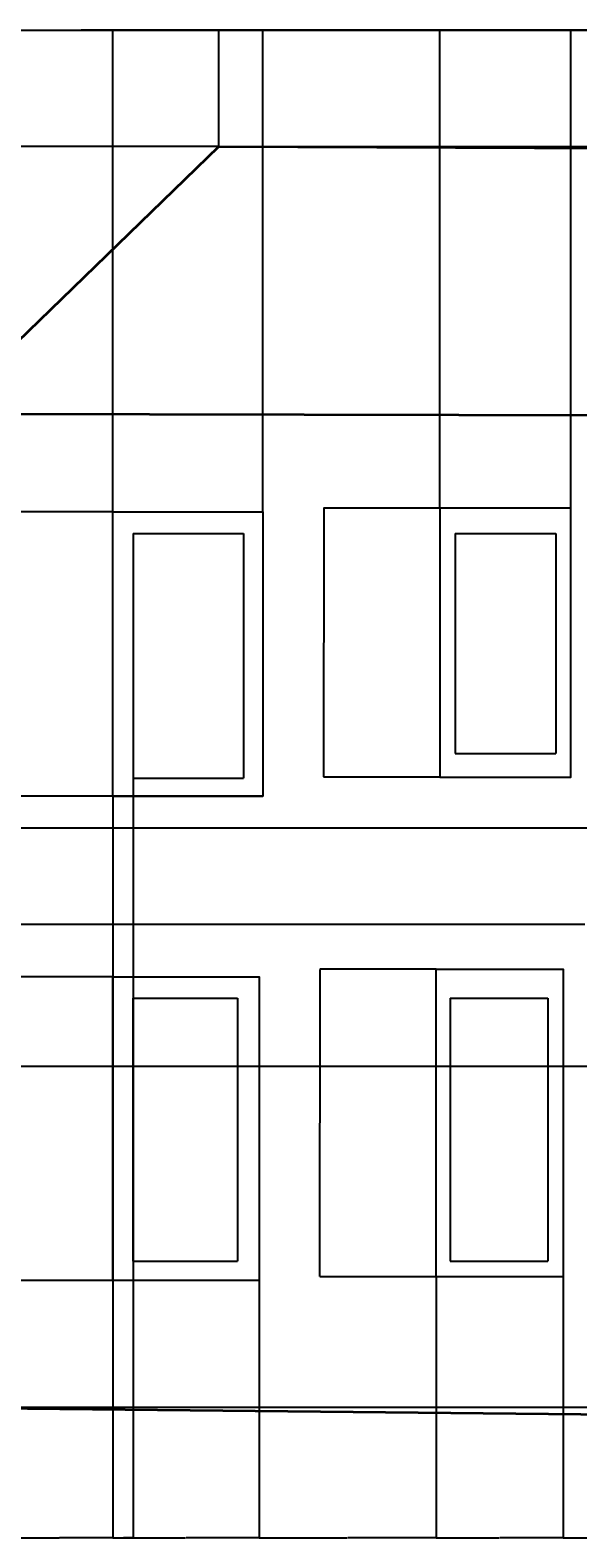
# Model space of a CAD drawing. Units: millimetres. Extents: x 1119 to 4262, y 854 to 2737.
# Tile 3 of 5: x 2434 to 3118, y 854 to 2737. Entities that reach past the tile are written whole.
import ezdxf

# ---------------------------------------------------------------- set-up
doc = ezdxf.new("R2010")
doc.units = ezdxf.units.MM
for name, color, linetype, lineweight in [('A-ANNO-DIMS', 2, 'Continuous', 18), ('A-ELEV', 8, 'Continuous', 35), ('A-GLAZ', 4, 'Continuous', 25), ('A-ROOF', 1, 'Continuous', 35)]:
    doc.layers.add(name, color=color, linetype=linetype, lineweight=lineweight)
doc.styles.get("Standard").update_dxf_attribs({"font": 'arial.ttf'})
doc.dimstyles.get("Standard").update_dxf_attribs({"dimtxt": 0.18, "dimasz": 0.18, "dimexe": 0.18, "dimexo": 0.0625, "dimgap": 0.09, "dimtad": 0, "dimtih": 1, "dimtoh": 1, "dimdec": 4, "dimzin": 0, "dimdsep": 46, "dimtxsty": 'Standard', "dimcen": 0.09, "dimadec": 0, "dimazin": 0, "dimtfac": 1, "dimtdec": 4, "dimtofl": 0, "dimtmove": 0, "dimatfit": 3, "dimfxl": 1, "dimtolj": 1, "dimtzin": 0, "dimarcsym": 0})

# ---------------------------------------------------------------- blocks, each defined once
blk = doc.blocks.new('*D5')
at = {"layer": 'A-ANNO-DIMS', "color": 0, "lineweight": -2, "transparency": 16777216}
for p, q in [((2537.2, 1175.4), (2537.2, 854.2)), ((2403.9, 1016.1), (2403.9, 854.2)), ((2404.1, 854.4), (2470.2, 854.4)), ((2537, 854.4), (2470.9, 854.4))]:
    blk.add_line(p, q, dxfattribs=at)
at = {"layer": 'A-ANNO-DIMS', "color": 0, "transparency": 16777216}
for points in [[(2404.1, 854.4), (2404.1, 854.3), (2403.9, 854.4)], [(2537, 854.4), (2537, 854.3), (2537.2, 854.4)]]:
    blk.add_solid(points, dxfattribs=at)
at = {"layer": 'Defpoints', "color": 0, "transparency": 16777216}
for p in [(2537.2, 1175.4), (2403.9, 1016.2), (2537.2, 854.4)]:
    blk.add_point(p, dxfattribs=at)
at = {"layer": 'A-ANNO-DIMS', "color": 0, "transparency": 16777216, "insert": (2470.5, 854.4), "char_height": 0.18, "attachment_point": 5}
blk.add_mtext('\\A1;133.3', dxfattribs=at)
blk = doc.blocks.new('*D6')
at = {"layer": 'A-ANNO-DIMS', "color": 0, "lineweight": -2, "transparency": 16777216}
for p, q in [((2537.2, 1175.4), (2537.2, 854.2)), ((2719.7, 1175.4), (2719.7, 854.2)), ((2537.4, 854.4), (2628, 854.4)), ((2719.5, 854.4), (2628.9, 854.4))]:
    blk.add_line(p, q, dxfattribs=at)
at = {"layer": 'A-ANNO-DIMS', "color": 0, "transparency": 16777216}
for points in [[(2537.4, 854.4), (2537.4, 854.3), (2537.2, 854.4)], [(2719.5, 854.4), (2719.5, 854.3), (2719.7, 854.4)]]:
    blk.add_solid(points, dxfattribs=at)
at = {"layer": 'Defpoints', "color": 0, "transparency": 16777216}
for p in [(2537.2, 1175.4), (2719.7, 1175.4), (2719.7, 854.4)]:
    blk.add_point(p, dxfattribs=at)
at = {"layer": 'A-ANNO-DIMS', "color": 0, "transparency": 16777216, "insert": (2628.5, 854.4), "char_height": 0.18, "attachment_point": 5}
blk.add_mtext('\\A1;182.52', dxfattribs=at)
blk = doc.blocks.new('*D7')
at = {"layer": 'A-ANNO-DIMS', "color": 0, "lineweight": -2, "transparency": 16777216}
for p, q in [((2719.7, 1175.4), (2719.7, 854.2)), ((2940.7, 1180.2), (2940.7, 854.2)), ((2719.9, 854.4), (2829.7, 854.4)), ((2940.5, 854.4), (2830.7, 854.4))]:
    blk.add_line(p, q, dxfattribs=at)
at = {"layer": 'A-ANNO-DIMS', "color": 0, "transparency": 16777216}
for points in [[(2719.9, 854.4), (2719.9, 854.3), (2719.7, 854.4)], [(2940.5, 854.4), (2940.5, 854.3), (2940.7, 854.4)]]:
    blk.add_solid(points, dxfattribs=at)
at = {"layer": 'Defpoints', "color": 0, "transparency": 16777216}
for p in [(2719.7, 1175.4), (2940.7, 1180.2), (2940.7, 854.4)]:
    blk.add_point(p, dxfattribs=at)
at = {"layer": 'A-ANNO-DIMS', "color": 0, "transparency": 16777216, "insert": (2830.2, 854.4), "char_height": 0.18, "attachment_point": 5}
blk.add_mtext('\\A1;220.95', dxfattribs=at)
blk = doc.blocks.new('*D8')
at = {"layer": 'A-ANNO-DIMS', "color": 0, "lineweight": -2, "transparency": 16777216}
for p, q in [((2940.7, 1180.2), (2940.7, 854.2)), ((3099.2, 1180.2), (3099.2, 854.2)), ((2940.8, 854.4), (3019.5, 854.4)), ((3099, 854.4), (3020.3, 854.4))]:
    blk.add_line(p, q, dxfattribs=at)
at = {"layer": 'A-ANNO-DIMS', "color": 0, "transparency": 16777216}
for points in [[(2940.8, 854.4), (2940.8, 854.3), (2940.7, 854.4)], [(3099, 854.4), (3099, 854.3), (3099.2, 854.4)]]:
    blk.add_solid(points, dxfattribs=at)
at = {"layer": 'Defpoints', "color": 0, "transparency": 16777216}
for p in [(2940.7, 1180.2), (3099.2, 1180.2), (3099.2, 854.4)]:
    blk.add_point(p, dxfattribs=at)
at = {"layer": 'A-ANNO-DIMS', "color": 0, "transparency": 16777216, "insert": (3019.9, 854.4), "char_height": 0.18, "attachment_point": 5}
blk.add_mtext('\\A1;158.5', dxfattribs=at)
blk = doc.blocks.new('*D9')
at = {"layer": 'A-ANNO-DIMS', "color": 0, "lineweight": -2, "transparency": 16777216}
for p, q in [((3099.2, 1180.2), (3099.2, 854.2)), ((3174.6, 1008), (3174.6, 854.2)), ((3099.4, 854.4), (3136.5, 854.4)), ((3174.4, 854.4), (3137.3, 854.4))]:
    blk.add_line(p, q, dxfattribs=at)
at = {"layer": 'A-ANNO-DIMS', "color": 0, "transparency": 16777216}
for points in [[(3099.4, 854.4), (3099.4, 854.3), (3099.2, 854.4)], [(3174.4, 854.4), (3174.4, 854.3), (3174.6, 854.4)]]:
    blk.add_solid(points, dxfattribs=at)
at = {"layer": 'Defpoints', "color": 0, "transparency": 16777216}
for p in [(3099.2, 1180.2), (3174.6, 1008.1), (3174.6, 854.4)]:
    blk.add_point(p, dxfattribs=at)
at = {"layer": 'A-ANNO-DIMS', "color": 0, "transparency": 16777216, "insert": (3136.9, 854.4), "char_height": 0.18, "attachment_point": 5}
blk.add_mtext('\\A1;75.38', dxfattribs=at)
blk = doc.blocks.new('*D13')
at = {"layer": 'A-ANNO-DIMS', "color": 0, "lineweight": -2, "transparency": 16777216}
for p, q in [((1264.4, 1028.3), (1264.4, 2737.1)), ((1264.5, 2737), (2690.1, 2737)), ((4116.6, 2737), (2691, 2737)), ((4116.8, 2249.8), (4116.8, 2737.1))]:
    blk.add_line(p, q, dxfattribs=at)
at = {"layer": 'A-ANNO-DIMS', "color": 0, "transparency": 16777216}
for points in [[(1264.5, 2737), (1264.5, 2736.9), (1264.4, 2737)], [(4116.6, 2737), (4116.6, 2736.9), (4116.8, 2737)]]:
    blk.add_solid(points, dxfattribs=at)
at = {"layer": 'Defpoints', "color": 0, "transparency": 16777216}
for p in [(4116.8, 2737), (4116.8, 2249.7), (1264.4, 1028.2)]:
    blk.add_point(p, dxfattribs=at)
at = {"layer": 'A-ANNO-DIMS', "color": 0, "transparency": 16777216, "insert": (2690.6, 2737), "char_height": 0.18, "attachment_point": 5}
blk.add_mtext('\\A1;2852.4', dxfattribs=at)
blk = doc.blocks.new('*D14')
at = {"layer": 'A-ANNO-DIMS', "color": 0, "lineweight": -2, "transparency": 16777216}
for p, q in [((2325.6, 2257.9), (2325.6, 2737.1)), ((2325.8, 2737), (2497.3, 2737)), ((2669.4, 2737), (2497.9, 2737)), ((2669.6, 2592), (2669.6, 2737.1))]:
    blk.add_line(p, q, dxfattribs=at)
at = {"layer": 'A-ANNO-DIMS', "color": 0, "transparency": 16777216}
for points in [[(2325.8, 2737), (2325.8, 2736.9), (2325.6, 2737)], [(2669.4, 2737), (2669.4, 2736.9), (2669.6, 2737)]]:
    blk.add_solid(points, dxfattribs=at)
at = {"layer": 'Defpoints', "color": 0, "transparency": 16777216}
for p in [(2669.6, 2737), (2669.6, 2592), (2325.6, 2257.9)]:
    blk.add_point(p, dxfattribs=at)
at = {"layer": 'A-ANNO-DIMS', "color": 0, "transparency": 16777216, "insert": (2497.6, 2737), "char_height": 0.18, "attachment_point": 5}
blk.add_mtext('\\A1;344', dxfattribs=at)
blk = doc.blocks.new('*D15')
at = {"layer": 'A-ANNO-DIMS', "color": 0, "lineweight": -2, "transparency": 16777216}
for p, q in [((2669.6, 2592), (2669.6, 2737.1)), ((2669.8, 2737), (3309.4, 2737)), ((3949.9, 2737), (3310.3, 2737)), ((3950, 2586.1), (3950, 2737.1))]:
    blk.add_line(p, q, dxfattribs=at)
at = {"layer": 'A-ANNO-DIMS', "color": 0, "transparency": 16777216}
for points in [[(2669.8, 2737), (2669.8, 2736.9), (2669.6, 2737)], [(3949.9, 2737), (3949.9, 2736.9), (3950, 2737)]]:
    blk.add_solid(points, dxfattribs=at)
at = {"layer": 'Defpoints', "color": 0, "transparency": 16777216}
for p in [(3950, 2737), (2669.6, 2592), (3950, 2586)]:
    blk.add_point(p, dxfattribs=at)
at = {"layer": 'A-ANNO-DIMS', "color": 0, "transparency": 16777216, "insert": (3309.8, 2737), "char_height": 0.18, "attachment_point": 5}
blk.add_mtext('\\A1;1280.4', dxfattribs=at)
blk = doc.blocks.new('*D25')
at = {"layer": 'A-ANNO-DIMS', "color": 0, "lineweight": -2, "transparency": 16777216}
for p, q in [((2537.2, 2135.6), (2537.2, 2737.1)), ((2537.4, 2737), (2630.4, 2737)), ((2724.3, 2737), (2631.3, 2737)), ((2724.5, 2135.6), (2724.5, 2737.1))]:
    blk.add_line(p, q, dxfattribs=at)
at = {"layer": 'A-ANNO-DIMS', "color": 0, "transparency": 16777216}
for points in [[(2537.4, 2737), (2537.4, 2736.9), (2537.2, 2737)], [(2724.3, 2737), (2724.3, 2736.9), (2724.5, 2737)]]:
    blk.add_solid(points, dxfattribs=at)
at = {"layer": 'Defpoints', "color": 0, "transparency": 16777216}
for p in [(2724.5, 2737), (2537.2, 2135.5), (2724.5, 2135.5)]:
    blk.add_point(p, dxfattribs=at)
at = {"layer": 'A-ANNO-DIMS', "color": 0, "transparency": 16777216, "insert": (2630.9, 2737), "char_height": 0.18, "attachment_point": 5}
blk.add_mtext('\\A1;187.33', dxfattribs=at)
blk = doc.blocks.new('*D26')
at = {"layer": 'A-ANNO-DIMS', "color": 0, "lineweight": -2, "transparency": 16777216}
for p, q in [((2724.5, 2135.6), (2724.5, 2737.1)), ((2724.7, 2737), (2834.5, 2737)), ((2945.3, 2737), (2835.5, 2737)), ((2945.5, 2140.4), (2945.5, 2737.1))]:
    blk.add_line(p, q, dxfattribs=at)
at = {"layer": 'A-ANNO-DIMS', "color": 0, "transparency": 16777216}
for points in [[(2724.7, 2737), (2724.7, 2736.9), (2724.5, 2737)], [(2945.3, 2737), (2945.3, 2736.9), (2945.5, 2737)]]:
    blk.add_solid(points, dxfattribs=at)
at = {"layer": 'Defpoints', "color": 0, "transparency": 16777216}
for p in [(2945.5, 2737), (2724.5, 2135.5), (2945.5, 2140.3)]:
    blk.add_point(p, dxfattribs=at)
at = {"layer": 'A-ANNO-DIMS', "color": 0, "transparency": 16777216, "insert": (2835, 2737), "char_height": 0.18, "attachment_point": 5}
blk.add_mtext('\\A1;220.95', dxfattribs=at)
blk = doc.blocks.new('*D27')
at = {"layer": 'A-ANNO-DIMS', "color": 0, "lineweight": -2, "transparency": 16777216}
for p, q in [((2945.5, 2140.4), (2945.5, 2737.1)), ((2945.6, 2737), (3026.7, 2737)), ((3108.6, 2737), (3027.5, 2737)), ((3108.8, 2140.4), (3108.8, 2737.1))]:
    blk.add_line(p, q, dxfattribs=at)
at = {"layer": 'A-ANNO-DIMS', "color": 0, "transparency": 16777216}
for points in [[(2945.6, 2737), (2945.6, 2736.9), (2945.5, 2737)], [(3108.6, 2737), (3108.6, 2736.9), (3108.8, 2737)]]:
    blk.add_solid(points, dxfattribs=at)
at = {"layer": 'Defpoints', "color": 0, "transparency": 16777216}
for p in [(3108.8, 2737), (2945.5, 2140.3), (3108.8, 2140.3)]:
    blk.add_point(p, dxfattribs=at)
at = {"layer": 'A-ANNO-DIMS', "color": 0, "transparency": 16777216, "insert": (3027.1, 2737), "char_height": 0.18, "attachment_point": 5}
blk.add_mtext('\\A1;163.3', dxfattribs=at)
blk = doc.blocks.new('*D28')
at = {"layer": 'A-ANNO-DIMS', "color": 0, "lineweight": -2, "transparency": 16777216}
for p, q in [((2562.7, 1803), (2562.7, 854.2)), ((2537.2, 1780.2), (2537.2, 854.2)), ((2537.4, 854.4), (2549.6, 854.4)), ((2562.5, 854.4), (2550.4, 854.4))]:
    blk.add_line(p, q, dxfattribs=at)
at = {"layer": 'A-ANNO-DIMS', "color": 0, "transparency": 16777216}
for points in [[(2537.4, 854.4), (2537.4, 854.3), (2537.2, 854.4)], [(2562.5, 854.4), (2562.5, 854.3), (2562.7, 854.4)]]:
    blk.add_solid(points, dxfattribs=at)
at = {"layer": 'Defpoints', "color": 0, "transparency": 16777216}
for p in [(2562.7, 1803.1), (2537.2, 1780.3), (2562.7, 854.4)]:
    blk.add_point(p, dxfattribs=at)
at = {"layer": 'A-ANNO-DIMS', "color": 0, "transparency": 16777216, "insert": (2550, 854.4), "char_height": 0.18, "attachment_point": 5}
blk.add_mtext('\\A1;25.54', dxfattribs=at)
blk = doc.blocks.new('*D29')
at = {"layer": 'A-ANNO-DIMS', "color": 0, "lineweight": -2, "transparency": 16777216}
for p, q in [((2940.6, 1564.3), (2795.5, 1564.3)), ((2795.7, 1564.1), (2795.7, 1372.4)), ((2795.7, 1180.4), (2795.7, 1372.1)), ((2940.6, 1180.2), (2795.5, 1180.2))]:
    blk.add_line(p, q, dxfattribs=at)
at = {"layer": 'A-ANNO-DIMS', "color": 0, "transparency": 16777216}
for points in [[(2795.6, 1564.1), (2795.7, 1564.1), (2795.7, 1564.3)], [(2795.6, 1180.4), (2795.7, 1180.4), (2795.7, 1180.2)]]:
    blk.add_solid(points, dxfattribs=at)
at = {"layer": 'Defpoints', "color": 0, "transparency": 16777216}
for p in [(2795.7, 1564.3), (2940.7, 1564.3), (2940.7, 1180.2)]:
    blk.add_point(p, dxfattribs=at)
at = {"layer": 'A-ANNO-DIMS', "color": 0, "transparency": 16777216, "insert": (2795.7, 1372.3), "char_height": 0.18, "attachment_point": 5}
blk.add_mtext('\\A1;384', dxfattribs=at)
blk = doc.blocks.new('*D30')
at = {"layer": 'A-ANNO-DIMS', "color": 0, "lineweight": -2, "transparency": 16777216}
for p, q in [((2945.4, 2140.3), (2800.3, 2140.3)), ((2800.5, 2140.1), (2800.5, 1972.5)), ((2800.5, 1804.5), (2800.5, 1972.1)), ((2945.4, 1804.3), (2800.3, 1804.3))]:
    blk.add_line(p, q, dxfattribs=at)
at = {"layer": 'A-ANNO-DIMS', "color": 0, "transparency": 16777216}
for points in [[(2800.4, 2140.1), (2800.5, 2140.1), (2800.5, 2140.3)], [(2800.4, 1804.5), (2800.5, 1804.5), (2800.5, 1804.3)]]:
    blk.add_solid(points, dxfattribs=at)
at = {"layer": 'Defpoints', "color": 0, "transparency": 16777216}
for p in [(2800.5, 2140.3), (2945.5, 2140.3), (2945.5, 1804.3)]:
    blk.add_point(p, dxfattribs=at)
at = {"layer": 'A-ANNO-DIMS', "color": 0, "transparency": 16777216, "insert": (2800.5, 1972.3), "char_height": 0.18, "attachment_point": 5}
blk.add_mtext('\\A1;336', dxfattribs=at)
blk = doc.blocks.new('*D31')
at = {"layer": 'A-ANNO-DIMS', "color": 0, "lineweight": -2, "transparency": 16777216}
for p, q in [((2537.1, 1175.4), (1119.2, 1175.4)), ((1119.4, 1175.3), (1119.4, 1096)), ((1119.4, 1016.4), (1119.4, 1095.6)), ((2403.8, 1016.2), (1119.2, 1016.2))]:
    blk.add_line(p, q, dxfattribs=at)
at = {"layer": 'A-ANNO-DIMS', "color": 0, "transparency": 16777216}
for points in [[(1119.3, 1175.3), (1119.4, 1175.3), (1119.4, 1175.4)], [(1119.3, 1016.4), (1119.4, 1016.4), (1119.4, 1016.2)]]:
    blk.add_solid(points, dxfattribs=at)
at = {"layer": 'Defpoints', "color": 0, "transparency": 16777216}
for p in [(1119.4, 1175.4), (2537.2, 1175.4), (2403.9, 1016.2)]:
    blk.add_point(p, dxfattribs=at)
at = {"layer": 'A-ANNO-DIMS', "color": 0, "transparency": 16777216, "insert": (1119.4, 1095.8), "char_height": 0.18, "attachment_point": 5}
blk.add_mtext('\\A1;159.26', dxfattribs=at)
blk = doc.blocks.new('*D32')
at = {"layer": 'A-ANNO-DIMS', "color": 0, "lineweight": -2, "transparency": 16777216}
for p, q in [((2537.1, 1554.7), (1119.2, 1554.7)), ((1119.4, 1554.5), (1119.4, 1365.2)), ((1119.4, 1175.6), (1119.4, 1364.9)), ((2537.1, 1175.4), (1119.2, 1175.4))]:
    blk.add_line(p, q, dxfattribs=at)
at = {"layer": 'A-ANNO-DIMS', "color": 0, "transparency": 16777216}
for points in [[(1119.3, 1554.5), (1119.4, 1554.5), (1119.4, 1554.7)], [(1119.3, 1175.6), (1119.4, 1175.6), (1119.4, 1175.4)]]:
    blk.add_solid(points, dxfattribs=at)
at = {"layer": 'Defpoints', "color": 0, "transparency": 16777216}
for p in [(1119.4, 1554.7), (2537.2, 1554.7), (2537.2, 1175.4)]:
    blk.add_point(p, dxfattribs=at)
at = {"layer": 'A-ANNO-DIMS', "color": 0, "transparency": 16777216, "insert": (1119.4, 1365.1), "char_height": 0.18, "attachment_point": 5}
blk.add_mtext('\\A1;379.2', dxfattribs=at)
blk = doc.blocks.new('*D33')
at = {"layer": 'A-ANNO-DIMS', "color": 0, "lineweight": -2, "transparency": 16777216}
for p, q in [((2537.1, 1780.3), (1119.2, 1780.3)), ((1119.4, 1780.1), (1119.4, 1667.7)), ((1119.4, 1554.9), (1119.4, 1667.3)), ((2537.1, 1554.7), (1119.2, 1554.7))]:
    blk.add_line(p, q, dxfattribs=at)
at = {"layer": 'A-ANNO-DIMS', "color": 0, "transparency": 16777216}
for points in [[(1119.3, 1780.1), (1119.4, 1780.1), (1119.4, 1780.3)], [(1119.3, 1554.9), (1119.4, 1554.9), (1119.4, 1554.7)]]:
    blk.add_solid(points, dxfattribs=at)
at = {"layer": 'Defpoints', "color": 0, "transparency": 16777216}
for p in [(1119.4, 1780.3), (2537.2, 1780.3), (2537.2, 1554.7)]:
    blk.add_point(p, dxfattribs=at)
at = {"layer": 'A-ANNO-DIMS', "color": 0, "transparency": 16777216, "insert": (1119.4, 1667.5), "char_height": 0.18, "attachment_point": 5}
blk.add_mtext('\\A1;225.6', dxfattribs=at)
blk = doc.blocks.new('*D34')
at = {"layer": 'A-ANNO-DIMS', "color": 0, "lineweight": -2, "transparency": 16777216}
for p, q in [((2537.1, 2135.5), (1119.2, 2135.5)), ((1119.4, 2135.3), (1119.4, 1958.1)), ((1119.4, 1780.5), (1119.4, 1957.7)), ((2537.1, 1780.3), (1119.2, 1780.3))]:
    blk.add_line(p, q, dxfattribs=at)
at = {"layer": 'A-ANNO-DIMS', "color": 0, "transparency": 16777216}
for points in [[(1119.3, 2135.3), (1119.4, 2135.3), (1119.4, 2135.5)], [(1119.3, 1780.5), (1119.4, 1780.5), (1119.4, 1780.3)]]:
    blk.add_solid(points, dxfattribs=at)
at = {"layer": 'Defpoints', "color": 0, "transparency": 16777216}
for p in [(1119.4, 2135.5), (2537.2, 2135.5), (2537.2, 1780.3)]:
    blk.add_point(p, dxfattribs=at)
at = {"layer": 'A-ANNO-DIMS', "color": 0, "transparency": 16777216, "insert": (1119.4, 1957.9), "char_height": 0.18, "attachment_point": 5}
blk.add_mtext('\\A1;355.2', dxfattribs=at)
blk = doc.blocks.new('*D35')
at = {"layer": 'A-ANNO-DIMS', "color": 0, "lineweight": -2, "transparency": 16777216}
for p, q in [((2416.9, 2257.7), (1119.2, 2257.7)), ((1119.4, 2257.5), (1119.4, 2196.8)), ((1119.4, 2135.7), (1119.4, 2196.4)), ((2537.1, 2135.5), (1119.2, 2135.5))]:
    blk.add_line(p, q, dxfattribs=at)
at = {"layer": 'A-ANNO-DIMS', "color": 0, "transparency": 16777216}
for points in [[(1119.3, 2257.5), (1119.4, 2257.5), (1119.4, 2257.7)], [(1119.3, 2135.7), (1119.4, 2135.7), (1119.4, 2135.5)]]:
    blk.add_solid(points, dxfattribs=at)
at = {"layer": 'Defpoints', "color": 0, "transparency": 16777216}
for p in [(1119.4, 2257.7), (2417, 2257.7), (2537.2, 2135.5)]:
    blk.add_point(p, dxfattribs=at)
at = {"layer": 'A-ANNO-DIMS', "color": 0, "transparency": 16777216, "insert": (1119.4, 2196.6), "char_height": 0.18, "attachment_point": 5}
blk.add_mtext('\\A1;122.15', dxfattribs=at)
blk = doc.blocks.new('*D36')
at = {"layer": 'A-ANNO-DIMS', "color": 0, "lineweight": -2, "transparency": 16777216}
for p, q in [((2669.5, 2592), (1119.2, 2592)), ((1119.4, 2591.8), (1119.4, 2425)), ((1119.4, 2257.8), (1119.4, 2424.6)), ((2416.9, 2257.7), (1119.2, 2257.7))]:
    blk.add_line(p, q, dxfattribs=at)
at = {"layer": 'A-ANNO-DIMS', "color": 0, "transparency": 16777216}
for points in [[(1119.3, 2591.8), (1119.4, 2591.8), (1119.4, 2592)], [(1119.3, 2257.8), (1119.4, 2257.8), (1119.4, 2257.7)]]:
    blk.add_solid(points, dxfattribs=at)
at = {"layer": 'Defpoints', "color": 0, "transparency": 16777216}
for p in [(1119.4, 2592), (2669.6, 2592), (2417, 2257.7)]:
    blk.add_point(p, dxfattribs=at)
at = {"layer": 'A-ANNO-DIMS', "color": 0, "transparency": 16777216, "insert": (1119.4, 2424.8), "char_height": 0.18, "attachment_point": 5}
blk.add_mtext('\\A1;334.3', dxfattribs=at)
blk = doc.blocks.new('*D44')
at = {"layer": 'A-ANNO-DIMS', "color": 0, "lineweight": -2, "transparency": 16777216}
for p, q in [((2669.7, 2592), (4262, 2592)), ((4261.8, 2591.8), (4261.8, 2565.4)), ((4261.8, 2538.6), (4261.8, 2565)), ((3586.7, 2538.4), (4262, 2538.4))]:
    blk.add_line(p, q, dxfattribs=at)
at = {"layer": 'A-ANNO-DIMS', "color": 0, "transparency": 16777216}
for points in [[(4261.8, 2591.8), (4261.8, 2591.8), (4261.8, 2592)], [(4261.8, 2538.6), (4261.8, 2538.6), (4261.8, 2538.4)]]:
    blk.add_solid(points, dxfattribs=at)
at = {"layer": 'Defpoints', "color": 0, "transparency": 16777216}
for p in [(2669.6, 2592), (4261.8, 2592), (3586.7, 2538.4)]:
    blk.add_point(p, dxfattribs=at)
at = {"layer": 'A-ANNO-DIMS', "color": 0, "transparency": 16777216, "insert": (4261.8, 2565.2), "char_height": 0.18, "attachment_point": 5}
blk.add_mtext('\\A1;53.57', dxfattribs=at)
blk = doc.blocks.new('*D67')
at = {"layer": 'A-ANNO-DIMS', "color": 0, "lineweight": -2, "transparency": 16777216}
for p, q in [((3217.2, 1740.6), (1119.2, 1740.6)), ((1119.4, 1740.4), (1119.4, 1680.5)), ((1119.4, 1620.3), (1119.4, 1680.1)), ((3126.2, 1620.1), (1119.2, 1620.1))]:
    blk.add_line(p, q, dxfattribs=at)
at = {"layer": 'A-ANNO-DIMS', "color": 0, "transparency": 16777216}
for points in [[(1119.3, 1740.4), (1119.4, 1740.4), (1119.4, 1740.6)], [(1119.3, 1620.3), (1119.4, 1620.3), (1119.4, 1620.1)]]:
    blk.add_solid(points, dxfattribs=at)
at = {"layer": 'Defpoints', "color": 0, "transparency": 16777216}
for p in [(1119.4, 1740.6), (3217.3, 1740.6), (3126.3, 1620.1)]:
    blk.add_point(p, dxfattribs=at)
at = {"layer": 'A-ANNO-DIMS', "color": 0, "transparency": 16777216, "insert": (1119.4, 1680.3), "char_height": 0.18, "attachment_point": 5}
blk.add_mtext('\\A1;120.48', dxfattribs=at)
blk = doc.blocks.new('*D78')
at = {"layer": 'A-ANNO-DIMS', "color": 0, "lineweight": -2, "transparency": 16777216}
for p, q in [((2297.6, 1443.4), (4262, 1443.4)), ((4261.8, 1443.2), (4261.8, 1230.6)), ((4261.8, 1017.5), (4261.8, 1230.2)), ((2293.1, 1017.4), (4262, 1017.4))]:
    blk.add_line(p, q, dxfattribs=at)
at = {"layer": 'A-ANNO-DIMS', "color": 0, "transparency": 16777216}
for points in [[(4261.8, 1443.2), (4261.8, 1443.2), (4261.8, 1443.4)], [(4261.8, 1017.5), (4261.8, 1017.5), (4261.8, 1017.4)]]:
    blk.add_solid(points, dxfattribs=at)
at = {"layer": 'Defpoints', "color": 0, "transparency": 16777216}
for p in [(2297.6, 1443.4), (4261.8, 1443.4), (2293.1, 1017.4)]:
    blk.add_point(p, dxfattribs=at)
at = {"layer": 'A-ANNO-DIMS', "color": 0, "transparency": 16777216, "insert": (4261.8, 1230.4), "char_height": 0.18, "attachment_point": 5}
blk.add_mtext('\\A1;426.06', dxfattribs=at)

msp = doc.modelspace()

# ---------------------------------------------------------------- linework, layer by layer
at = {"layer": 'A-ELEV'}
msp.add_line((1264.3595, 1028.2021), (4000.5454, 999.3572), dxfattribs=at)
at = {"layer": 'A-GLAZ'}
for p, q in [((2562.7277, 2108.3713), (2700.3205, 2108.3713)), ((2562.7277, 2108.3713), (2562.7277, 1803.0534)), ((2700.3205, 2108.3713), (2700.3205, 1803.0534)), ((2964.664, 2108.3713), (2964.664, 1833.5547)), ((2964.664, 2108.3713), (3090.0836, 2108.3713)), ((3090.0836, 2108.3713), (3090.0836, 1833.5547)), ((2964.664, 1833.5547), (3090.0836, 1833.5547)), ((2562.7277, 1803.0534), (2700.3205, 1803.0534)), ((2537.1892, 1780.2865), (2724.5165, 1780.2865)), ((2562.3624, 1528.1532), (2692.6754, 1528.1532)), ((2562.3624, 1528.1532), (2562.3624, 1199.5851)), ((2692.6754, 1528.1532), (2692.6754, 1199.5851)), ((2958.0835, 1528.1532), (3080.0277, 1528.1532)), ((2958.0835, 1528.1532), (2958.0835, 1199.5851)), ((3080.0277, 1528.1532), (3080.0277, 1199.5851)), ((2562.3624, 1199.5851), (2692.6754, 1199.5851)), ((2958.0835, 1199.5851), (3080.0277, 1199.5851))]:
    msp.add_line(p, q, dxfattribs=at)
for points in [[(2537.1892, 2135.5085), (2724.5165, 2135.5085), (2724.5165, 1780.2865), (2537.1892, 1780.2865)], [(3108.7776, 2140.3088), (2945.4666, 2140.3088), (2945.4666, 1804.288), (3108.7776, 1804.288)], [(2940.6634, 1564.2732), (3099.1711, 1564.2732), (3099.1711, 1180.2494), (2940.6634, 1180.2494)], [(2537.1892, 1554.6726), (2719.7132, 1554.6726), (2719.7132, 1175.4491), (2537.1892, 1175.4491)]]:
    msp.add_lwpolyline(points, close=True, dxfattribs=at)
at = {"layer": 'A-ROOF'}
for p, q in [((2325.6262, 2257.8652), (2669.6107, 2591.9672)), ((2669.6107, 2591.9672), (3950.0418, 2586.0154)), ((3323.0337, 2255.5648), (2325.6262, 2257.8652))]:
    msp.add_line(p, q, dxfattribs=at)

# ---------------------------------------------------------------- dimensions: what is measured, and where the dimension line sits
at = {"layer": 'A-ANNO-DIMS'}
for base, p1, p2, override, picture, middle in [((4116.7957, 2736.9672), (1264.3595, 1028.2021), (4116.7957, 2249.7378), {"dimdec": 1, "dimlfac": 1, "dimrnd": 0, "dimzin": 0, "dimdsep": 46, "dimlunit": 2}, '*D13', (2690.5776, 2736.9672)), ((2669.6107, 2736.9672), (2325.6262, 2257.8652), (2669.6107, 2591.9672), {"dimdec": 0, "dimlfac": 1, "dimrnd": 0, "dimzin": 0, "dimdsep": 46, "dimlunit": 2}, '*D14', (2497.6185, 2736.9672)), ((2724.5165, 2736.9672), (2537.1892, 2135.5085), (2724.5165, 2135.5085), {"dimdec": 2, "dimlfac": 1, "dimrnd": 0, "dimzin": 0, "dimdsep": 46, "dimlunit": 2}, '*D25', (2630.8528, 2736.9672)), ((3950.0418, 2736.9672), (2669.6107, 2591.9672), (3950.0418, 2586.0154), {"dimdec": 1, "dimlfac": 1, "dimrnd": 0, "dimzin": 0, "dimdsep": 46, "dimlunit": 2}, '*D15', (3309.8263, 2736.9672)), ((2945.4666, 2736.9672), (2724.5165, 2135.5085), (2945.4666, 2140.3088), {"dimdec": 2, "dimlfac": 1, "dimrnd": 0, "dimzin": 0, "dimdsep": 46, "dimlunit": 2}, '*D26', (2834.9916, 2736.9672)), ((3108.7776, 2736.9672), (2945.4666, 2140.3088), (3108.7776, 2140.3088), {"dimdec": 1, "dimlfac": 1, "dimrnd": 0, "dimzin": 0, "dimdsep": 46, "dimlunit": 2}, '*D27', (3027.1221, 2736.9672)), ((2562.7277, 854.3572), (2537.1892, 1780.2865), (2562.7277, 1803.0534), {"dimdec": 2, "dimlfac": 1, "dimrnd": 0, "dimzin": 0, "dimdsep": 46, "dimlunit": 2}, '*D28', (2549.9584, 854.3572)), ((2537.1892, 854.3572), (2403.8929, 1016.1891), (2537.1892, 1175.4491), {"dimdec": 1, "dimlfac": 1, "dimrnd": 0, "dimzin": 0, "dimdsep": 46, "dimlunit": 2}, '*D5', (2470.5411, 854.3572)), ((2719.7132, 854.3572), (2537.1892, 1175.4491), (2719.7132, 1175.4491), {"dimdec": 2, "dimlfac": 1, "dimrnd": 0, "dimzin": 0, "dimdsep": 46, "dimlunit": 2}, '*D6', (2628.4512, 854.3572)), ((2940.6634, 854.3572), (2719.7132, 1175.4491), (2940.6634, 1180.2494), {"dimdec": 2, "dimlfac": 1, "dimrnd": 0, "dimzin": 0, "dimdsep": 46, "dimlunit": 2}, '*D7', (2830.1883, 854.3572)), ((3099.1711, 854.3572), (2940.6634, 1180.2494), (3099.1711, 1180.2494), {"dimdec": 1, "dimlfac": 1, "dimrnd": 0, "dimzin": 0, "dimdsep": 46, "dimlunit": 2}, '*D8', (3019.9172, 854.3572)), ((3174.5502, 854.3572), (3099.1711, 1180.2494), (3174.5502, 1008.0649), {"dimdec": 2, "dimlfac": 1, "dimrnd": 0, "dimzin": 0, "dimdsep": 46, "dimlunit": 2}, '*D9', (3136.8606, 854.3572))]:
    dim = msp.add_linear_dim(base=base, p1=p1, p2=p2, dimstyle='Standard', override=override, dxfattribs=at)
    dim.commit()
    dim.dimension.update_dxf_attribs({"geometry": picture, "text_midpoint": middle})
for base, p1, p2, override, picture, middle in [((1119.3595, 2591.9672), (2416.9805, 2257.6545), (2669.6107, 2591.9672), {"dimdec": 1, "dimlfac": 1, "dimrnd": 0, "dimzin": 0, "dimdsep": 46, "dimlunit": 2}, '*D36', (1119.3595, 2424.8109)), ((4261.7957, 2591.9672), (3586.6565, 2538.4005), (2669.6107, 2591.9672), {"dimdec": 2, "dimlfac": 1, "dimrnd": 0, "dimzin": 0, "dimdsep": 46, "dimlunit": 2}, '*D44', (4261.7957, 2565.1838)), ((1119.3595, 2257.6545), (2537.1892, 2135.5085), (2416.9805, 2257.6545), {"dimdec": 2, "dimlfac": 1, "dimrnd": 0, "dimzin": 0, "dimdsep": 46, "dimlunit": 2}, '*D35', (1119.3595, 2196.5815)), ((1119.3595, 2135.5085), (2537.1892, 1780.2865), (2537.1892, 2135.5085), {"dimdec": 1, "dimlfac": 1, "dimrnd": 0, "dimzin": 0, "dimdsep": 46, "dimlunit": 2}, '*D34', (1119.3595, 1957.8975)), ((2800.4666, 2140.3088), (2945.4666, 1804.288), (2945.4666, 2140.3088), {"dimdec": 0, "dimlfac": 1, "dimrnd": 0, "dimzin": 0, "dimdsep": 46, "dimlunit": 2}, '*D30', (2800.4666, 1972.2984)), ((1119.3595, 1780.2865), (2537.1892, 1554.6726), (2537.1892, 1780.2865), {"dimdec": 1, "dimlfac": 1, "dimrnd": 0, "dimzin": 0, "dimdsep": 46, "dimlunit": 2}, '*D33', (1119.3595, 1667.4795)), ((1119.3595, 1740.5658), (3126.2541, 1620.0857), (3217.2823, 1740.5658), {"dimdec": 2, "dimlfac": 1, "dimrnd": 0, "dimzin": 0, "dimdsep": 46, "dimlunit": 2}, '*D67', (1119.3595, 1680.3258)), ((2795.6634, 1564.2732), (2940.6634, 1180.2494), (2940.6634, 1564.2732), {"dimdec": 0, "dimlfac": 1, "dimrnd": 0, "dimzin": 0, "dimdsep": 46, "dimlunit": 2}, '*D29', (2795.6634, 1372.2613)), ((1119.3595, 1554.6726), (2537.1892, 1175.4491), (2537.1892, 1554.6726), {"dimdec": 1, "dimlfac": 1, "dimrnd": 0, "dimzin": 0, "dimdsep": 46, "dimlunit": 2}, '*D32', (1119.3595, 1365.0608)), ((4261.7957, 1443.4126), (2293.0699, 1017.3574), (2297.5614, 1443.4126), {"dimdec": 2, "dimlfac": 1, "dimrnd": 0, "dimzin": 0, "dimdsep": 46, "dimlunit": 2}, '*D78', (4261.7957, 1230.385)), ((1119.3595, 1175.4491), (2403.8929, 1016.1891), (2537.1892, 1175.4491), {"dimdec": 2, "dimlfac": 1, "dimrnd": 0, "dimzin": 0, "dimdsep": 46, "dimlunit": 2}, '*D31', (1119.3595, 1095.8191))]:
    dim = msp.add_linear_dim(base=base, p1=p1, p2=p2, angle=90, dimstyle='Standard', override=override, dxfattribs=at)
    dim.commit()
    dim.dimension.update_dxf_attribs({"geometry": picture, "text_midpoint": middle})

doc.saveas('drawing.dxf')
